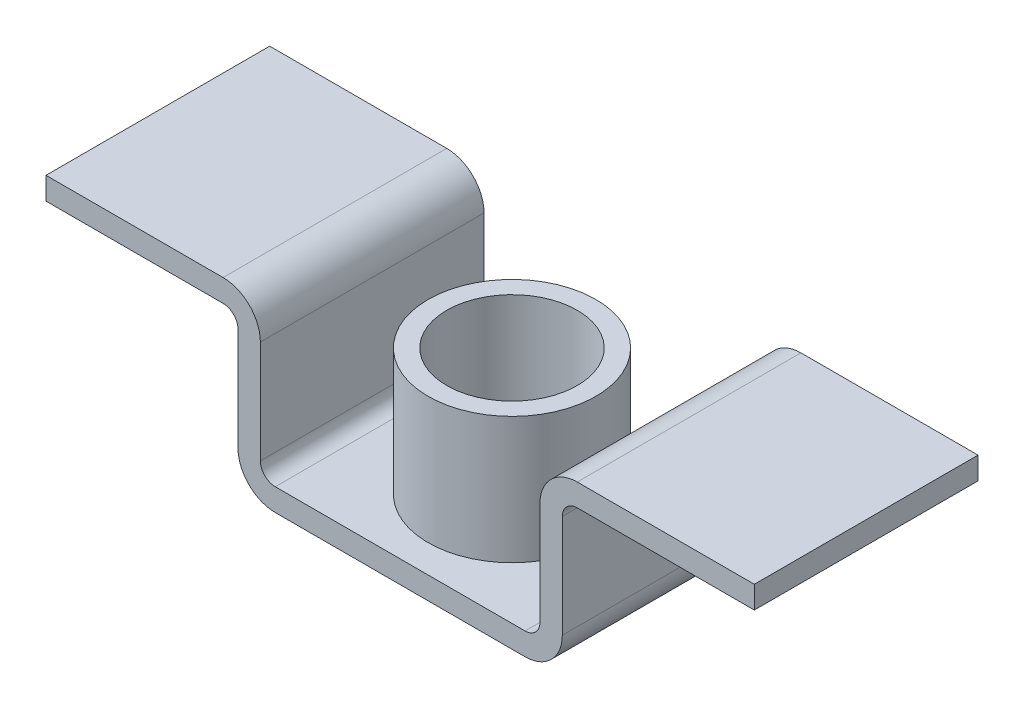
from build123d import *

# Parameters (mm, degrees)
FORMED_BRACKET_BODY_DEPTH = 150
BOSS_TUBE_SKETCH_R        = 112.5
BOSS_TUBE_SKETCH_R_2      = 87.5
BOSS_TUBE_225X170_DEPTH   = 170
BASE_HOLE_75_REACH        = 541.805
BASE_HOLE_SKETCH_R        = 37.5


with BuildPart() as part:
    # Bracket Profile Sketch → Formed Bracket Body (new, symmetric)
    with BuildSketch(Plane.XY):
        with BuildLine():
            Line((-475, 0), (-237.5, 0))
            ThreePointArc((-237.5, 0), (-202.144660941, -14.644660941), (-187.5, -50))
            Line((-187.5, -50), (-187.5, -188))
            ThreePointArc((-187.5, -188), (-181.642135624, -202.142135624), (-167.5, -208))
            Line((-167.5, -208), (167.5, -208))
            ThreePointArc((167.5, -208), (181.642135624, -202.142135624), (187.5, -188))
            Line((187.5, -188), (187.5, -50))
            ThreePointArc((187.5, -50), (202.144660941, -14.644660941), (237.5, 0))
            Line((237.5, 0), (475, 0))
            Line((475, 0), (475, -30))
            Line((475, -30), (237.5, -30))
            ThreePointArc((237.5, -30), (223.357864376, -35.857864376), (217.5, -50))
            Line((217.5, -50), (217.5, -188))
            ThreePointArc((217.5, -188), (202.855339059, -223.355339059), (167.5, -238))
            Line((167.5, -238), (-167.5, -238))
            ThreePointArc((-167.5, -238), (-202.855339059, -223.355339059), (-217.5, -188))
            Line((-217.5, -188), (-217.5, -50))
            ThreePointArc((-217.5, -50), (-223.357864376, -35.857864376), (-237.5, -30))
            Line((-237.5, -30), (-475, -30))
            Line((-475, -30), (-475, 0))
        make_face()
    extrude(amount=FORMED_BRACKET_BODY_DEPTH, both=True)

    # Boss Tube Sketch → Boss Tube Ø225x170 (add)
    with BuildSketch(Plane(origin=(0, -208, 0), x_dir=(1, 0, 0), z_dir=(0, 1, 0))):
        with Locations(Location((0, 0, 0), (0, 0, 180))):
            Circle(BOSS_TUBE_SKETCH_R)
        with Locations(Location((0, 0, 0), (0, 0, 180))):
            Circle(BOSS_TUBE_SKETCH_R_2, mode=Mode.SUBTRACT)
    extrude(amount=BOSS_TUBE_225X170_DEPTH)

    # Base Hole Sketch → Base Hole Ø75 (cut, up to next)
    with BuildSketch(Plane(origin=(0, -208, 0), x_dir=(1, 0, 0), z_dir=(0, 1, 0)), mode=Mode.PRIVATE) as base_hole_75_sk1:
        with Locations(Location((0, 0, 0), (0, 0, 180))):
            Circle(BASE_HOLE_SKETCH_R)
    base_hole_75_tool1 = extrude(base_hole_75_sk1.sketch, amount=-BASE_HOLE_75_REACH, mode=Mode.PRIVATE) & part.part
    add(base_hole_75_tool1.solids().sort_by_distance((0, -208, 0))[0], mode=Mode.SUBTRACT)


solid = part.part
